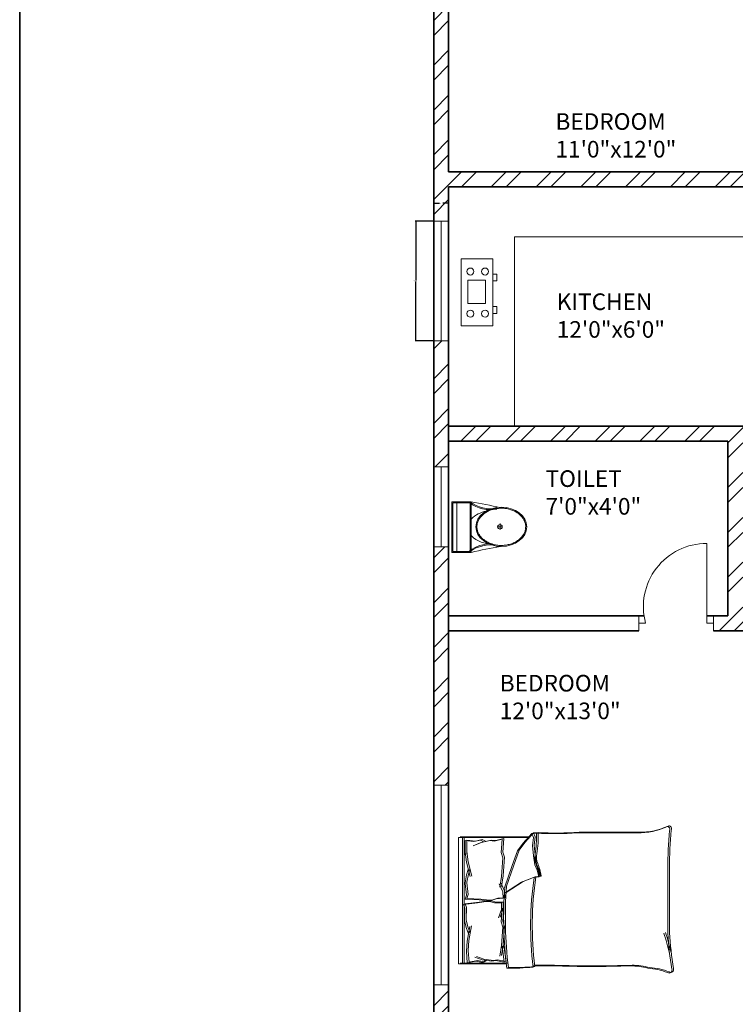
# Model space of a CAD drawing. Units: inches. Extents: x 1962 to 2771, y 1245 to 2660.
# Tile 2 of 114: x 1962 to 2177, y 1534 to 1831. Entities that reach past the tile are written whole.
import ezdxf

# ---------------------------------------------------------------- set-up
doc = ezdxf.new("R2010")
doc.units = ezdxf.units.IN
for name, color, linetype, lineweight in [('A-ANNO-DIMS', 2, 'Continuous', 18), ('A-ANNO-TTLB', 7, 'Continuous', 35), ('A-AREA-IDEN', 7, 'Continuous', 18), ('A-DOOR', 3, 'Continuous', 18), ('A-EQPM', 8, 'Continuous', 18), ('A-FLOR-CASE', 8, 'Continuous', 18), ('A-FLOR-FIXT', 8, 'Continuous', 18), ('A-FURN', 8, 'Continuous', 13), ('A-GLAZ', 4, 'Continuous', 18), ('A-WALL', 7, 'Continuous', 35), ('A-WALL-PATT', 252, 'Continuous', 13)]:
    doc.layers.add(name, color=color, linetype=linetype, lineweight=lineweight)
doc.styles.get("Standard").update_dxf_attribs({"font": 'arial.ttf'})
doc.dimstyles.get("Standard").update_dxf_attribs({"dimtxt": 0.18, "dimasz": 0.18, "dimexe": 0.18, "dimexo": 0.0625, "dimgap": 0.09, "dimtad": 0, "dimtih": 1, "dimtoh": 1, "dimdec": 4, "dimzin": 0, "dimdsep": 46, "dimtxsty": 'Standard', "dimcen": 0.09, "dimadec": 0, "dimazin": 0, "dimtfac": 1, "dimtdec": 4, "dimtofl": 0, "dimtmove": 0, "dimatfit": 3, "dimfxl": 1, "dimtolj": 1, "dimtzin": 0, "dimarcsym": 0})

# ---------------------------------------------------------------- blocks, each defined once
blk = doc.blocks.new('A$C31115884')
for p, q in [((258, 466), (258, 523)), ((283, 498), (223, 498)), ((0, 200), (0, 0)), ((520, 200), (0, 200)), ((10, 190), (10, 10)), ((510, 190), (10, 190)), ((510, 10), (510, 190)), ((520, 0), (520, 200)), ((510, 54), (0, 54)), ((10, 10), (510, 10)), ((0, 0), (520, 0))]:
    blk.add_line(p, q)
blk.add_circle((256, 496), 23.6)
for centre, radius, start, end in [((2778, -205), 2807, 165.4549, 171.7133), ((-295, 403), 365, 324.2091, 9.3499), ((-295, 403), 375, 324.2091, 9.3499), ((139, 406), 293, 315.8436, 2.6563), ((806, 403), 375, 179.2036, 215.7909), ((806, 403), 365, 170.6501, 215.7909), ((3237, 905), 2807, 188.2867, 194.5451), ((384, 406), 293, 190.2774, 224.1564)]:
    blk.add_arc(centre, radius, start, end)
blk.add_ellipse((256, 510), major_axis=(0, -261), ratio=0.772727)
blk.add_open_spline([(256, 259), (263, 259), (270, 260), (288, 262), (299, 265), (320, 273), (330, 278), (350, 291), (360, 299), (378, 316), (386, 326), (402, 347), (409, 358), (421, 383), (427, 395), (436, 422), (440, 436), (445, 465), (447, 480), (448, 509), (448, 524), (445, 553), (443, 568), (436, 596), (432, 610), (422, 636), (416, 649), (402, 672), (395, 683), (379, 703), (370, 712), (351, 728), (341, 735), (321, 746), (310, 751), (289, 757), (278, 759), (256, 761), (245, 761), (223, 757), (212, 754), (191, 746), (181, 741), (161, 728), (151, 720), (133, 703), (125, 693), (110, 672), (103, 660), (90, 636), (85, 623), (76, 596), (72, 582), (67, 553), (66, 538), (64, 509), (65, 494), (68, 465), (70, 450), (77, 422), (81, 408), (91, 382), (97, 370), (111, 346), (118, 335), (135, 316), (144, 307), (162, 291), (172, 284), (193, 273), (203, 269), (225, 262), (236, 260), (250, 259), (253, 259), (256, 259)], degree=3, knots=[0, 0, 0, 0, 0.110105, 0.110105, 0.285049, 0.285049, 0.459994, 0.459994, 0.634938, 0.634938, 0.809882, 0.809882, 0.984827, 0.984827, 1.159771, 1.159771, 1.334715, 1.334715, 1.50966, 1.50966, 1.684604, 1.684604, 1.859549, 1.859549, 2.034493, 2.034493, 2.209437, 2.209437, 2.384382, 2.384382, 2.559326, 2.559326, 2.73427, 2.73427, 2.909215, 2.909215, 3.084159, 3.084159, 3.259103, 3.259103, 3.434048, 3.434048, 3.608992, 3.608992, 3.783936, 3.783936, 3.958881, 3.958881, 4.133825, 4.133825, 4.30877, 4.30877, 4.483714, 4.483714, 4.658658, 4.658658, 4.833603, 4.833603, 5.008547, 5.008547, 5.183491, 5.183491, 5.358436, 5.358436, 5.53338, 5.53338, 5.708324, 5.708324, 5.883269, 5.883269, 6.058213, 6.058213, 6.233158, 6.233158, 6.283185, 6.283185, 6.283185, 6.283185])
blk = doc.blocks.new('BED-PLAN')
for p, q in [((22.05, 42.03), (19.47, 39.08)), ((22.05, 42.02), (19.47, 39.08)), ((22.56, 42.21), (19.98, 39.26)), ((22.56, 42.21), (19.98, 39.26)), ((23.44, 42.09), (22.05, 42.03, 3.08)), ((23.44, 42.09), (22.05, 42.02, 3.08)), ((22.55, 40.8), (22.05, 42.03)), ((22.55, 40.8), (22.05, 42.02)), ((23.95, 42.27), (22.56, 42.21, 3.08)), ((23.95, 42.27), (22.56, 42.21, 3.08)), ((23.06, 40.98), (22.56, 42.21)), ((23.06, 40.98), (22.56, 42.21)), ((0, 40.75), (21.15, 40.75)), ((0, 40.75), (21.15, 40.75)), ((0, 2.76), (0, 40.75)), ((0.51, 40.93), (21.66, 40.93)), ((0.51, 40.93), (21.66, 40.93)), ((1.22, 2.76), (1.22, 40.75)), ((1.22, 2.76), (1.22, 40.75)), ((1.73, 2.95), (1.73, 40.93)), ((1.73, 2.95), (1.73, 40.93)), ((2.03, 39.83), (1.96, 35.54)), ((2.03, 39.83), (1.96, 35.54)), ((2.03, 39.83), (4.58, 39.53)), ((2.03, 39.83), (4.58, 39.53)), ((2.54, 40.02), (2.46, 35.72)), ((2.54, 40.02), (2.46, 35.72)), ((2.54, 40.02), (5.09, 39.72)), ((2.54, 40.02), (5.09, 39.72)), ((6.56, 39.2), (4.43, 38.26)), ((6.56, 39.2), (4.43, 38.26)), ((4.58, 39.53), (6.63, 40.01)), ((4.58, 39.53), (6.63, 40.01)), ((7.07, 39.38), (4.94, 38.44)), ((7.07, 39.38), (4.94, 38.44)), ((5.09, 39.72), (7.14, 40.19)), ((5.09, 39.72), (7.14, 40.19)), ((9.4, 39.83), (6.56, 39.2)), ((9.4, 39.83), (6.56, 39.2)), ((6.63, 40.01), (7.46, 39.6)), ((6.63, 40.01), (7.46, 39.6)), ((9.91, 40.02), (7.07, 39.38)), ((9.91, 40.02), (7.07, 39.38)), ((7.14, 40.19), (7.97, 39.78)), ((7.14, 40.19), (7.97, 39.78)), ((10.68, 39.68), (9.4, 39.83)), ((10.68, 39.68), (9.4, 39.83)), ((11.19, 39.87), (9.91, 40.02)), ((11.19, 39.87), (9.91, 40.02)), ((13.17, 40.3), (10.68, 39.68)), ((13.17, 40.3), (10.68, 39.68)), ((13.68, 40.48), (11.19, 39.87)), ((13.68, 40.48), (11.19, 39.87)), ((12.85, 36.22), (13.17, 40.3)), ((12.85, 36.22), (13.17, 40.3)), ((13.36, 36.4), (13.68, 40.48)), ((13.36, 36.4), (13.68, 40.48)), ((19.47, 39.08), (17.75, 36.74)), ((19.47, 39.08), (17.75, 36.74)), ((19.98, 39.26), (18.26, 36.92)), ((19.98, 39.26), (18.26, 36.92)), ((22.3, 38.34), (22.55, 40.8)), ((22.3, 38.34), (22.55, 40.8)), ((22.81, 38.52), (23.06, 40.98)), ((22.81, 38.52), (23.06, 40.98)), ((23.06, 35.45), (22.81, 38.52)), ((23.06, 35.44), (22.81, 38.52)), ((1.96, 35.54), (2.02, 36.34)), ((1.96, 35.54), (2.02, 36.34)), ((2.02, 36.34), (2.44, 33.32)), ((2.02, 36.34), (2.44, 33.32)), ((2.46, 35.72), (2.53, 36.52)), ((2.46, 35.72), (2.53, 36.52)), ((2.53, 36.52), (2.95, 33.5)), ((2.53, 36.52), (2.95, 33.5)), ((13.3, 34.66), (12.85, 36.22)), ((13.3, 34.66), (12.85, 36.22)), ((13.8, 34.84), (13.36, 36.4)), ((13.8, 34.84), (13.36, 36.4)), ((17.75, 36.74), (16.15, 32.31)), ((17.75, 36.74), (16.15, 32.31)), ((18.26, 36.92), (16.66, 32.49)), ((18.26, 36.92), (16.66, 32.49)), ((22.55, 35.26), (22.3, 38.34)), ((22.55, 35.26), (22.3, 38.34)), ((2.44, 33.32), (3.52, 29.01)), ((2.44, 33.32), (3.52, 29.01)), ((2.95, 33.5), (4.02, 29.19)), ((2.95, 33.5), (4.02, 29.19)), ((12.95, 29.09), (13.3, 34.66)), ((12.95, 29.09), (13.3, 34.66)), ((13.46, 29.27), (13.8, 34.84)), ((13.46, 29.27), (13.8, 34.84)), ((22.92, 32.56), (22.55, 35.26)), ((22.92, 32.55), (22.55, 35.26)), ((23.42, 32.74), (23.06, 35.45)), ((23.42, 32.74), (23.06, 35.44)), ((24.16, 31.14), (23.42, 32.74)), ((24.16, 31.14), (23.42, 32.74)), ((2.92, 31.16), (2.45, 29.52)), ((2.92, 31.16), (2.45, 29.52)), ((2.96, 29.7), (2.52, 27.37)), ((2.96, 29.7), (2.52, 27.37)), ((3.43, 31.34), (2.96, 29.7)), ((3.43, 31.34), (2.96, 29.7)), ((16.15, 32.31), (13.82, 25.68)), ((16.15, 32.31), (13.82, 25.68)), ((16.66, 32.49), (14.33, 25.86)), ((16.66, 32.49), (14.33, 25.86)), ((23.65, 30.95), (22.92, 32.56)), ((23.65, 30.95), (22.92, 32.55)), ((24.15, 28.99), (23.65, 30.95)), ((24.15, 28.98), (23.65, 30.95)), ((24.65, 29.17), (24.16, 31.14)), ((24.65, 29.17), (24.16, 31.14)), ((62.99, 11.98), (62.99, 31.54)), ((62.99, 11.97), (62.99, 31.54)), ((63.5, 12.16), (63.5, 31.72)), ((63.5, 12.16), (63.5, 31.72)), ((2.45, 29.52), (2.02, 27.19)), ((2.45, 29.52), (2.02, 27.19)), ((2.02, 27.19), (2.03, 26.94)), ((2.02, 27.19), (2.03, 26.93)), ((2.03, 26.94), (2.37, 23.42)), ((2.03, 26.93), (2.37, 23.42)), ((2.52, 27.37), (2.54, 27.12)), ((2.52, 27.37), (2.54, 27.12)), ((2.54, 27.12), (2.88, 23.6)), ((2.54, 27.12), (2.88, 23.6)), ((13.31, 24.44), (12.28, 26.89)), ((13.31, 24.44), (12.28, 26.88)), ((12.42, 25.89), (12.95, 29.09)), ((12.42, 25.89), (12.95, 29.09)), ((13.81, 24.63), (12.79, 27.07)), ((13.81, 24.63), (12.79, 27.07)), ((12.93, 26.07), (13.46, 29.27)), ((12.93, 26.07), (13.46, 29.27)), ((13.82, 24.05), (18.98, 27.38)), ((13.82, 24.05), (18.98, 27.38)), ((14.33, 24.24), (19.49, 27.57)), ((14.33, 24.24), (19.49, 27.57)), ((18.98, 27.38), (22.55, 28.74)), ((18.98, 27.38), (22.55, 28.74)), ((19.49, 27.57), (23.06, 28.92)), ((19.49, 27.57), (23.06, 28.92)), ((22.55, 28.74), (24.15, 28.99)), ((22.55, 28.74), (24.15, 28.98)), ((23.06, 28.92), (24.65, 29.17)), ((23.06, 28.92), (24.65, 29.17)), ((13.43, 22.49), (13.31, 24.44)), ((13.43, 22.49), (13.31, 24.44)), ((13.94, 22.68), (13.81, 24.63)), ((13.94, 22.68), (13.81, 24.63)), ((1.49, 20.65), (5.74, 21.11)), ((1.49, 20.65), (5.74, 21.11)), ((2.37, 23.42), (1.98, 22.24)), ((2.37, 23.42), (1.98, 22.24)), ((1.98, 22.24), (6.25, 22.05)), ((1.98, 22.24), (6.25, 22.05)), ((1.99, 20.84), (6.25, 21.3)), ((1.99, 20.84), (6.25, 21.3)), ((2.45, 19.69), (1.99, 20.84)), ((2.45, 19.69), (1.99, 20.84)), ((2.88, 23.6), (2.49, 22.42)), ((2.88, 23.6), (2.49, 22.42)), ((2.49, 22.42), (6.76, 22.23)), ((2.49, 22.42), (6.76, 22.23)), ((5.74, 21.11), (8.27, 21.57)), ((5.74, 21.11), (8.27, 21.57)), ((6.25, 22.05), (8.81, 21.75)), ((6.25, 22.05), (8.81, 21.75)), ((6.25, 21.3), (8.78, 21.76)), ((6.25, 21.3), (8.78, 21.76)), ((6.76, 22.23), (9.31, 21.93)), ((6.76, 22.23), (9.31, 21.93)), ((8.27, 21.57), (9.3, 21.57)), ((8.27, 21.57), (9.3, 21.57)), ((8.78, 21.76), (9.81, 21.76)), ((8.78, 21.76), (9.81, 21.76)), ((8.81, 21.75), (9.84, 21.81)), ((8.81, 21.75), (9.84, 21.81)), ((9.3, 21.57), (10.8, 21.11)), ((9.3, 21.57), (10.8, 21.11)), ((9.31, 21.93), (10.35, 21.99)), ((9.31, 21.93), (10.35, 21.99)), ((9.81, 21.76), (11.3, 21.3)), ((9.81, 21.76), (11.3, 21.3)), ((9.84, 21.81), (11.3, 22.36)), ((9.84, 21.81), (11.3, 22.36)), ((10.35, 21.99), (11.81, 22.54)), ((10.35, 21.99), (11.81, 22.54)), ((10.8, 21.11), (12.93, 21.11)), ((10.8, 21.11), (12.93, 21.11)), ((11.3, 22.36), (13.43, 22.49)), ((11.3, 22.36), (13.43, 22.49)), ((11.3, 21.3), (13.44, 21.3)), ((11.3, 21.3), (13.44, 21.3)), ((11.81, 22.54), (13.94, 22.68)), ((11.81, 22.54), (13.94, 22.68)), ((12.93, 21.11), (12.93, 19.16)), ((12.93, 21.11), (12.93, 19.16)), ((13.44, 21.3), (13.44, 19.34)), ((13.44, 21.3), (13.44, 19.34)), ((1.95, 19.51), (1.49, 20.65)), ((1.95, 19.51), (1.49, 20.65)), ((1.83, 15.97), (1.95, 19.51)), ((1.83, 15.97), (1.95, 19.51)), ((2.34, 16.15), (2.45, 19.69)), ((2.34, 16.15), (2.45, 19.69)), ((12.93, 19.16), (12.06, 16.66)), ((12.93, 19.16), (12.06, 16.66)), ((13.44, 19.34), (12.57, 16.84)), ((13.44, 19.34), (12.57, 16.84)), ((12.85, 15.41), (13.17, 19.49)), ((12.85, 15.41), (13.17, 19.49)), ((13.36, 15.59), (13.68, 19.67)), ((13.36, 15.59), (13.68, 19.67)), ((1.83, 15.72), (1.83, 15.97)), ((1.83, 15.72), (1.83, 15.97)), ((2.41, 13.42), (1.83, 15.72)), ((2.41, 13.42), (1.83, 15.72)), ((2.34, 15.9), (2.34, 16.15)), ((2.34, 15.9), (2.34, 16.15)), ((2.91, 13.6), (2.34, 15.9)), ((2.91, 13.6), (2.34, 15.9)), ((13.3, 13.85), (12.85, 15.41)), ((13.3, 13.85), (12.85, 15.41)), ((13.8, 14.03), (13.36, 15.59)), ((13.8, 14.03), (13.36, 15.59)), ((2.98, 11.81), (2.41, 13.42)), ((2.98, 11.81), (2.41, 13.42)), ((2.64, 9.63), (3.44, 13.99)), ((2.64, 9.63), (3.44, 13.99)), ((3.49, 11.99), (2.91, 13.6)), ((3.49, 11.99), (2.91, 13.6)), ((3.14, 9.81), (3.95, 14.17)), ((3.14, 9.81), (3.95, 14.17)), ((12.95, 8.28), (13.3, 13.85)), ((12.95, 8.28), (13.3, 13.85)), ((13.46, 8.46), (13.8, 14.03)), ((13.46, 8.46), (13.8, 14.03)), ((2.41, 6.59), (2.64, 9.63)), ((2.41, 6.59), (2.64, 9.63)), ((2.91, 6.77), (3.14, 9.81)), ((2.91, 6.77), (3.14, 9.81)), ((2.39, 6.5), (2.41, 6.59)), ((2.39, 6.5), (2.41, 6.59)), ((2.65, 3.1), (2.39, 6.5)), ((2.65, 3.1), (2.39, 6.5)), ((2.9, 6.68), (2.91, 6.77)), ((2.9, 6.68), (2.91, 6.77)), ((3.16, 3.28), (2.9, 6.68)), ((3.16, 3.28), (2.9, 6.68)), ((12.42, 5.07), (12.95, 8.28)), ((12.42, 5.07), (12.95, 8.28)), ((12.93, 5.26), (13.46, 8.46)), ((12.93, 5.26), (13.46, 8.46)), ((12.95, 8.28), (13.21, 7.38)), ((12.95, 8.28), (13.21, 7.38)), ((13.21, 7.38), (13.78, 3.33)), ((13.21, 7.38), (13.78, 3.33)), ((13.46, 8.46), (13.72, 7.56)), ((13.46, 8.46), (13.72, 7.56)), ((13.72, 7.56), (14.29, 3.51)), ((13.72, 7.56), (14.29, 3.51)), ((2.64, 3.1), (5.16, 3.56)), ((2.64, 3.1), (5.16, 3.56)), ((3.14, 3.28), (5.67, 3.74)), ((3.14, 3.28), (5.67, 3.74)), ((7.12, 4.02), (4.93, 4.82)), ((7.12, 4.02), (4.93, 4.82)), ((5.16, 3.56), (7.23, 3.21)), ((5.16, 3.56), (7.23, 3.21)), ((7.63, 4.2), (5.44, 5)), ((7.63, 4.2), (5.44, 5)), ((5.67, 3.74), (7.74, 3.39)), ((5.67, 3.74), (7.74, 3.39)), ((9.99, 3.56), (7.12, 4.02)), ((9.99, 3.56), (7.12, 4.02)), ((7.23, 3.21), (8.04, 3.67)), ((7.23, 3.21), (8.04, 3.67)), ((10.5, 3.74), (7.63, 4.2)), ((10.5, 3.74), (7.63, 4.2)), ((7.74, 3.39), (8.55, 3.85)), ((7.74, 3.39), (8.55, 3.85)), ((11.26, 3.79), (9.99, 3.56)), ((11.26, 3.79), (9.99, 3.56)), ((11.76, 3.97), (10.5, 3.74)), ((11.76, 3.97), (10.5, 3.74)), ((13.78, 3.33), (11.26, 3.79)), ((13.78, 3.33), (11.26, 3.79)), ((14.29, 3.51), (11.76, 3.97)), ((14.29, 3.51), (11.76, 3.97)), ((14.4, 2.76), (0, 2.76)), ((14.4, 2.76), (0, 2.76)), ((14.9, 2.95), (0.51, 2.95)), ((14.9, 2.95), (0.51, 2.95))]:
    blk.add_line(p, q)
for centre, radius, start, end in [((-5.29, 40.8), 28.76, 349.8763, 2.5657), ((-5.29, 40.8), 28.76, 349.8763, 2.5657), ((28.87, 144.88), 102.94, 266.9791, 273.8365), ((28.87, 144.88), 102.94, 266.9791, 273.8365), ((-4.78, 40.98), 28.76, 349.8763, 2.5657), ((-4.78, 40.98), 28.76, 349.8763, 2.5657), ((29.37, 145.06), 102.94, 266.9791, 273.8365), ((29.37, 145.06), 102.94, 266.9791, 273.8365), ((53.91, -3583.94), 3626.16, 90.00217, 90.28689), ((53.91, -3583.94), 3626.16, 90.00217, 90.28689), ((54.42, -3583.75), 3626.16, 90.00217, 90.28689), ((54.42, -3583.75), 3626.16, 90.00217, 90.28689), ((54.58, 60.54), 18.33, 267.4714, 296.4681), ((54.58, 60.54), 18.33, 267.4714, 296.4681), ((55.09, 60.72), 18.33, 267.4714, 296.4681), ((55.09, 60.72), 18.33, 267.4714, 296.4681), ((62.69, 43.25), 0.876, 332.6588, 86.02), ((62.69, 43.25), 0.876, 332.6588, 86.02), ((168.74, 32.71), 105.75, 174.4998, 180.6351), ((168.74, 32.71), 105.75, 174.4998, 180.6351), ((63.2, 43.43), 0.876, 332.6588, 86.02), ((63.2, 43.43), 0.876, 332.6588, 86.02), ((169.24, 32.89), 105.75, 174.4998, 180.6351), ((169.24, 32.89), 105.75, 174.4998, 180.6351), ((27.87, 34.77), 4.95, 168.6608, 203.7384), ((27.87, 34.77), 4.95, 168.6608, 203.7384), ((28.38, 34.95), 4.95, 168.6608, 203.7384), ((28.38, 34.95), 4.95, 168.6608, 203.7384), ((1.18, 24.77), 23.57, 10.6617, 19.8806), ((1.18, 24.76), 23.57, 10.6617, 19.8806), ((1.69, 24.95), 23.57, 10.6617, 19.8806), ((1.69, 24.95), 23.57, 10.6617, 19.8806), ((124.25, 14.12), 102.56, 171.7845, 186.9006), ((124.25, 14.11), 102.56, 171.7845, 186.9006), ((124.76, 14.3), 102.56, 171.7845, 186.9006), ((124.76, 14.3), 102.56, 171.7845, 186.9006), ((24.2, 29.12), 0.147, 250.2464, 1.1377), ((24.2, 29.12), 0.147, 250.2464, 1.1377), ((24.7, 29.3), 0.147, 250.2464, 1.1377), ((24.7, 29.3), 0.147, 250.2464, 1.1377), ((144.71, 16.98), 131.13, 176.0865, 186.7821), ((144.71, 16.98), 131.13, 176.0865, 186.7821), ((145.22, 17.16), 131.13, 176.0865, 186.7821), ((145.22, 17.16), 131.13, 176.0865, 186.7821), ((-18.85, -13.69), 84.62, 13.3832, 17.7053), ((-18.85, -13.69), 84.62, 13.3832, 17.7053), ((-18.34, -13.51), 84.62, 13.3832, 17.7053), ((-18.34, -13.51), 84.62, 13.3832, 17.7053), ((159.64, 17.03), 96.78, 182.9958, 189.4091), ((159.64, 17.03), 96.78, 182.9958, 189.4091), ((160.15, 17.21), 96.78, 182.9958, 189.4091), ((160.15, 17.21), 96.78, 182.9958, 189.4091), ((15.97, 67.7), 66.22, 268.7218, 275.604), ((15.97, 67.7), 66.22, 268.7218, 275.604), ((16.48, 67.88), 66.22, 268.7218, 275.604), ((16.48, 67.88), 66.22, 268.7218, 275.604), ((24.78, -132.99), 135.22, 88.4762, 91.0082), ((24.78, -132.99), 135.22, 88.4762, 91.0082), ((25.29, -132.81), 135.22, 88.4762, 91.0082), ((25.29, -132.81), 135.22, 88.4762, 91.0082), ((40.23, 385.38), 383.38, 268.2277, 271.7185), ((40.23, 385.38), 383.38, 268.2277, 271.7185), ((40.74, 385.56), 383.38, 268.2277, 271.7185), ((40.74, 385.56), 383.38, 268.2277, 271.7185), ((51.28, -21.38), 23.56, 76.0648, 88.9113), ((51.28, -21.38), 23.56, 76.0648, 88.9113), ((51.79, -21.2), 23.56, 76.0648, 88.9113), ((51.79, -21.2), 23.56, 76.0648, 88.9113), ((55.86, -17.22), 18.73, 67.9751, 86.652), ((55.86, -17.22), 18.73, 67.9751, 86.652), ((56.37, -17.03), 18.73, 67.9751, 86.652), ((56.37, -17.03), 18.73, 67.9751, 86.652), ((63.37, 0.87), 0.866, 236.1736, 23.4781), ((63.37, 0.87), 0.866, 236.1736, 23.4781), ((63.87, 1.05), 0.866, 236.1736, 23.4781), ((63.87, 1.05), 0.866, 236.1736, 23.4781)]:
    blk.add_arc(centre, radius, start, end)
blk = doc.blocks.new('COOKTOP-4-BURNER')
for points in [[(0, 20.18), (9.48, 20.18), (9.48, 0), (0, 0)], [(9.48, 15.59), (10.71, 15.59), (10.71, 13.59), (9.48, 13.59)], [(2, 13.79), (7.26, 13.79), (7.26, 6.73), (2, 6.73)], [(9.48, 5.81), (10.71, 5.81), (10.71, 3.8), (9.48, 3.8)]]:
    blk.add_lwpolyline(points, close=True)
for centre in [(2.74, 16.38), (7.14, 16.38), (2.74, 3.71), (7.14, 3.71)]:
    blk.add_circle(centre, 1.05)
blk = doc.blocks.new('WIN-24IN-B')
for p, q in [((0, 24), (4.5, 24)), ((4.5, 24), (2.25, 24)), ((2.25, 24), (2.25, 0)), ((4.5, 0), (0, 0)), ((2.25, 0), (4.5, 0))]:
    blk.add_line(p, q)
blk = doc.blocks.new('WIN-60IN-B')
for p, q in [((0, 60), (4.5, 60)), ((4.5, 60), (2.25, 60)), ((2.25, 60), (2.25, 0)), ((4.5, 0), (0, 0)), ((2.25, 0), (4.5, 0))]:
    blk.add_line(p, q)
blk = doc.blocks.new('WIN-36IN-A')
for p, q in [((4.5, 36), (0, 36)), ((0, 36), (2.25, 36)), ((2.25, 36), (2.25, 0)), ((2.25, 0), (0, 0)), ((0, 0), (4.5, 0))]:
    blk.add_line(p, q)
blk = doc.blocks.new('*D26')
at = {"layer": 'A-ANNO-DIMS', "color": 0, "lineweight": -2, "transparency": 16777216}
for p, q in [((2086.24, 1769.99), (2080.73, 1769.99)), ((2080.91, 1769.81), (2080.91, 1752.17)), ((2080.91, 1734.17), (2080.91, 1751.81)), ((2086.24, 1733.99), (2080.73, 1733.99))]:
    blk.add_line(p, q, dxfattribs=at)
at = {"layer": 'A-ANNO-DIMS', "color": 0, "transparency": 16777216}
for points in [[(2080.88, 1769.81), (2080.94, 1769.81), (2080.91, 1769.99)], [(2080.88, 1734.17), (2080.94, 1734.17), (2080.91, 1733.99)]]:
    blk.add_solid(points, dxfattribs=at)
at = {"layer": 'Defpoints', "color": 0, "transparency": 16777216}
for p in [(2080.91, 1769.99), (2086.31, 1769.99), (2086.31, 1733.99)]:
    blk.add_point(p, dxfattribs=at)
at = {"layer": 'A-ANNO-DIMS', "color": 0, "transparency": 16777216, "insert": (2080.91, 1751.99), "char_height": 0.18, "attachment_point": 5}
blk.add_mtext('\\A1;W2A 36 TYP.', dxfattribs=at)
blk = doc.blocks.new('*D27')
at = {"layer": 'A-ANNO-DIMS', "color": 0, "lineweight": -2, "transparency": 16777216}
for p, q in [((2086.31, 1770.05), (2086.31, 1775.57)), ((2086.49, 1775.39), (2088.1, 1775.39)), ((2090.63, 1775.39), (2089.02, 1775.39)), ((2090.81, 1770.05), (2090.81, 1775.57))]:
    blk.add_line(p, q, dxfattribs=at)
at = {"layer": 'A-ANNO-DIMS', "color": 0, "transparency": 16777216}
for points in [[(2086.49, 1775.42), (2086.49, 1775.36), (2086.31, 1775.39)], [(2090.63, 1775.42), (2090.63, 1775.36), (2090.81, 1775.39)]]:
    blk.add_solid(points, dxfattribs=at)
at = {"layer": 'Defpoints', "color": 0, "transparency": 16777216}
for p in [(2090.81, 1775.39), (2086.31, 1769.99), (2090.81, 1769.99)]:
    blk.add_point(p, dxfattribs=at)
at = {"layer": 'A-ANNO-DIMS', "color": 0, "transparency": 16777216, "insert": (2088.56, 1775.39), "char_height": 0.18, "attachment_point": 5}
blk.add_mtext('\\A1;5 TYP.', dxfattribs=at)

msp = doc.modelspace()

# ---------------------------------------------------------------- hatches: boundary and pattern name
at = {"layer": 'A-WALL-PATT'}
h = msp.add_hatch(dxfattribs=at)
h.set_pattern_fill('ANSI32', color=256)
h.paths.add_polyline_path([(2090.8074, 2467.3437), (2141.6481, 2467.3437), (2141.6481, 2469.5937), (2141.6481, 2471.8437), (2086.3074, 2471.8437), (2086.3074, 2422.5333), (2090.8074, 2422.5333)])
h.paths.add_polyline_path([(2282.7664, 2471.8437), (2204.8982, 2471.8437), (2204.8982, 2467.3437), (2234.8074, 2467.3437), (2234.8074, 2311.3437), (2228.7492, 2311.3437), (2228.7492, 2306.8437), (2234.8074, 2306.8437), (2331.9227, 2306.8437), (2331.9227, 2309.0937), (2331.9227, 2311.3437), (2239.3074, 2311.3437), (2239.3074, 2467.3437), (2282.7664, 2467.3437), (2282.7664, 2469.5937)])
h.paths.add_polyline_path([(2471.4531, 2519.8437), (2552.011, 2519.8437), (2564.3996, 2519.8437), (2564.3996, 2511.1389), (2568.8996, 2511.1389), (2568.8996, 2524.3437), (2466.9531, 2524.3437), (2466.9531, 2471.8437), (2450.0749, 2471.8437), (2446.4672, 2471.8437), (2446.4672, 2467.3437), (2450.0749, 2467.3437), (2475.9988, 2467.3437), (2475.9988, 2469.5937), (2475.9988, 2471.8437), (2471.4531, 2471.8437)])
h.paths.add_polyline_path([(2575.2231, 2469.5937), (2575.2231, 2471.8437), (2568.8996, 2471.8437), (2568.8996, 2487.1389), (2564.3996, 2487.1389), (2564.3996, 2471.8437), (2556.511, 2471.8437), (2499.2904, 2471.8437), (2499.2904, 2467.3437), (2507.8074, 2467.3437), (2507.8074, 2311.3437), (2414.863, 2311.3437), (2414.863, 2306.8437), (2512.3074, 2306.8437), (2517.0114, 2306.8437), (2517.0114, 2309.0937), (2517.0114, 2311.3437), (2512.3074, 2311.3437), (2512.3074, 2467.3437), (2575.2231, 2467.3437)])
h.paths.add_polyline_path([(2660.8074, 2471.8437), (2600.9602, 2471.8437), (2600.9602, 2467.3437), (2656.3074, 2467.3437), (2656.3074, 2432.5704), (2660.8074, 2432.5704)])
h.paths.add_polyline_path([(2660.8074, 2372.5704), (2656.3074, 2372.5704), (2656.3074, 2311.3437), (2600.276, 2311.3437), (2600.276, 2309.0937), (2600.276, 2306.8437), (2656.3074, 2306.8437), (2656.3074, 2296.2593), (2660.8074, 2296.2593)])
h.paths.add_polyline_path([(2572.3074, 2306.8437), (2577.1385, 2306.8437), (2577.1385, 2311.3437), (2551.082, 2311.3437), (2551.082, 2306.8437), (2567.8074, 2306.8437), (2567.8074, 2258.8437), (2540.0574, 2258.8437), (2540.0574, 2256.5937), (2540.0574, 2254.3437), (2567.8074, 2254.3437), (2656.3074, 2254.3437), (2656.3074, 2236.9085), (2660.8074, 2236.9085), (2660.8074, 2272.2593), (2656.3074, 2272.2593), (2656.3074, 2258.8437), (2572.3074, 2258.8437)])
h.paths.add_polyline_path([(2512.3074, 2254.3437), (2518.8716, 2254.3437), (2518.8716, 2256.5937), (2518.8716, 2258.8437), (2507.8074, 2258.8437), (2507.8074, 2177.8437), (2567.8074, 2177.8437), (2567.8074, 2172.9628), (2572.3074, 2172.9628), (2572.3074, 2177.8437), (2656.3074, 2177.8437), (2656.3074, 2166.4846), (2660.8074, 2166.4846), (2660.8074, 2200.9085), (2656.3074, 2200.9085), (2656.3074, 2182.3437), (2512.3074, 2182.3437)])
h.paths.add_polyline_path([(2656.3074, 2129.8437), (2572.3074, 2129.8437), (2572.3074, 2150.3044), (2570.0574, 2150.3044), (2567.8074, 2150.3044), (2567.8074, 2129.8437), (2507.8074, 2129.8437), (2507.8074, 2116.3027), (2510.0574, 2116.3027), (2512.3074, 2116.3027), (2512.3074, 2125.3437), (2567.8074, 2125.3437), (2572.3074, 2125.3437), (2656.3074, 2125.3437)])
h.paths.add_polyline_path([(2090.8074, 2362.5333), (2086.3074, 2362.5333), (2086.3074, 2298.6242), (2090.8074, 2298.6242), (2090.8074, 2306.8437), (2174.8074, 2306.8437), (2174.8074, 2286.4178), (2179.3074, 2286.4178), (2179.3074, 2306.8437), (2192.8641, 2306.8437), (2192.8641, 2309.0937), (2192.8641, 2311.3437), (2090.8074, 2311.3437)])
h.paths.add_polyline_path([(2209.156, 2258.8437), (2179.3074, 2258.8437), (2179.3074, 2263.2236), (2177.0574, 2263.2236), (2174.8074, 2263.2236), (2174.8074, 2258.8437), (2090.8074, 2258.8437), (2090.8074, 2274.6242), (2086.3074, 2274.6242), (2086.3074, 2238.2967), (2088.5574, 2238.2967), (2090.8074, 2238.2967), (2090.8074, 2254.3437), (2209.156, 2254.3437)])
h.paths.add_polyline_path([(2090.8074, 2177.8437), (2234.8074, 2177.8437), (2234.8074, 2173.1428), (2239.3074, 2173.1428), (2239.3074, 2258.8437), (2230.8442, 2258.8437), (2230.8442, 2256.5937), (2230.8442, 2254.3437), (2234.8074, 2254.3437), (2234.8074, 2182.3437), (2090.8074, 2182.3437), (2090.8074, 2202.2967), (2086.3074, 2202.2967), (2086.3074, 2140.0389), (2090.8074, 2140.0389)])
h.paths.add_polyline_path([(2090.8074, 2080.0389), (2086.3074, 2080.0389), (2086.3074, 2033.8437), (2090.8074, 2033.8437)], flags=17)
h.paths.add_polyline_path([(2244.9405, 2033.8437), (2239.3074, 2033.8437), (2239.3074, 2142.0665), (2237.2592, 2142.0665), (2234.8074, 2142.0665), (2234.8074, 2033.8437), (2090.8074, 2033.8437), (2076.5204, 2033.8437), (2072.0204, 2033.8437), (2072.0204, 2000.4493), (2076.5204, 2000.4493), (2076.5204, 2029.3437), (2090.8074, 2029.3437), (2244.9405, 2029.3437), (2244.9405, 2031.5937)])
h.paths.add_polyline_path([(2234.8074, 1933.3437), (2076.5204, 1933.3437), (2076.5204, 1952.4493), (2074.2704, 1952.4493), (2072.0204, 1952.4493), (2072.0204, 1933.3437), (2072.0204, 1928.8437), (2234.8074, 1928.8437)])
h.paths.add_polyline_path([(2090.8074, 1928.8437), (2086.3074, 1928.8437), (2086.3074, 1906.5013), (2090.8074, 1906.5013)])
h.paths.add_polyline_path([(2090.8074, 1846.5013), (2086.3074, 1846.5013), (2086.3074, 1769.9917), (2088.5574, 1769.9917), (2090.8074, 1769.9917), (2090.8074, 1780.3437), (2234.8074, 1780.3437), (2234.8074, 1708.3437), (2230.3764, 1708.3437), (2230.3764, 1703.8437), (2239.3074, 1703.8437), (2239.3074, 1792.6669), (2237.0574, 1792.6669), (2234.8074, 1792.6669), (2234.8074, 1784.8437), (2090.8074, 1784.8437)])
h.paths.add_polyline_path([(2239.3074, 1928.8437), (2244.9405, 1928.8437), (2244.9405, 1931.0937), (2244.9405, 1933.3437), (2234.8074, 1933.3437), (2234.8074, 1928.8437), (2234.8074, 1825.5949), (2239.3074, 1825.5949)])
h.paths.add_polyline_path([(2148.0425, 1649.0937), (2148.0425, 1651.3437), (2090.8074, 1651.3437), (2090.8074, 1646.8437), (2148.0425, 1646.8437)], flags=0)
h.paths.add_polyline_path([(2207.5601, 1708.3437), (2090.8074, 1708.3437), (2090.8074, 1703.8437), (2174.8074, 1703.8437), (2174.8074, 1651.3437), (2170.4457, 1651.3437), (2170.4457, 1646.8437), (2195.9924, 1646.8437), (2195.9924, 1649.0937), (2195.9924, 1651.3437), (2179.3074, 1651.3437), (2179.3074, 1703.8437), (2207.5601, 1703.8437), (2207.5601, 1706.0937)])
h.paths.add_polyline_path([(2090.8074, 1733.9917), (2086.3074, 1733.9917), (2086.3074, 1696.1032), (2088.5574, 1696.1032), (2090.8074, 1696.1032)])
h.paths.add_polyline_path([(2090.8074, 1672.1032), (2086.3074, 1672.1032), (2086.3074, 1600.3335), (2090.8074, 1600.3335)])
h.paths.add_polyline_path([(2090.8074, 1540.3335), (2086.3074, 1540.3335), (2086.3074, 1486.3437), (2139.6766, 1486.3437), (2139.6766, 1490.8437), (2090.8074, 1490.8437)])
h.paths.add_polyline_path([(2302.3876, 1490.8437), (2239.3074, 1490.8437), (2239.3074, 1646.8437), (2335.9994, 1646.8437), (2335.9994, 1651.3437), (2229.884, 1651.3437), (2229.884, 1646.8437), (2234.8074, 1646.8437), (2234.8074, 1490.8437), (2202.7103, 1490.8437), (2202.7103, 1488.5937), (2202.7103, 1486.3437), (2275.0699, 1486.3437), (2275.0699, 1475.772), (2279.5699, 1475.772), (2279.5699, 1486.3437), (2302.3876, 1486.3437)])
h.paths.add_polyline_path([(2279.5699, 1451.772), (2275.0699, 1451.772), (2275.0699, 1438.3437), (2174.8074, 1438.3437), (2174.8074, 1486.3437), (2179.7922, 1486.3437), (2179.7922, 1490.8437), (2163.3585, 1490.8437), (2163.3585, 1488.5937), (2163.3585, 1486.3437), (2170.3074, 1486.3437), (2170.3074, 1433.8437), (2279.5699, 1433.8437)])
h.paths.add_polyline_path([(2427.2363, 1490.8437), (2375.8074, 1490.8437), (2375.8074, 1646.8437), (2381.6401, 1646.8437), (2381.6401, 1651.3437), (2365.887, 1651.3437), (2365.887, 1649.0937), (2365.887, 1646.8437), (2371.3074, 1646.8437), (2371.3074, 1490.8437), (2327.5627, 1490.8437), (2327.5627, 1488.5937), (2327.5627, 1486.3437), (2371.3074, 1486.3437), (2371.3074, 1433.8437), (2375.8074, 1433.8437), (2375.8074, 1486.3437), (2427.2363, 1486.3437)])
h.paths.add_polyline_path([(2512.3074, 1646.8437), (2519.4351, 1646.8437), (2519.4351, 1649.0937), (2519.4351, 1651.3437), (2507.8074, 1651.3437), (2416.0063, 1651.3437), (2416.0063, 1649.0937), (2416.0063, 1646.8437), (2507.8074, 1646.8437), (2507.8074, 1490.8437), (2497.0532, 1490.8437), (2497.0532, 1488.5937), (2497.0532, 1486.3437), (2574.9344, 1486.3437), (2574.9344, 1476.0181), (2579.4344, 1476.0181), (2579.4344, 1486.3437), (2584.4872, 1486.3437), (2584.3074, 1490.8437), (2512.3074, 1490.8437)])
h.paths.add_polyline_path([(2470.5091, 1486.3437), (2473.9767, 1486.3437), (2473.9767, 1490.8437), (2449.6605, 1490.8437), (2449.6605, 1488.5937), (2449.6605, 1486.3437), (2466.0091, 1486.3437), (2466.0091, 1433.8437), (2470.5091, 1433.8437), (2579.4344, 1433.8437), (2579.4344, 1452.0181), (2574.9344, 1452.0181), (2574.9344, 1438.3437), (2554.5091, 1438.3437), (2470.5091, 1438.3437)])
h.paths.add_polyline_path([(2656.3074, 1490.8437), (2611.86, 1490.8437), (2611.86, 1486.3437), (2656.3074, 1486.3437)])
h.paths.add_polyline_path([(2660.8074, 1532.7007), (2658.5574, 1532.7007), (2656.3074, 1532.7007), (2656.3074, 1486.3437), (2660.8074, 1486.3437)])
h.paths.add_polyline_path([(2660.8074, 1664.9663), (2656.3074, 1664.9663), (2656.3074, 1651.3437), (2602.2313, 1651.3437), (2602.2313, 1646.8437), (2656.3074, 1646.8437), (2656.3074, 1592.7007), (2660.8074, 1592.7007)])
h.paths.add_polyline_path([(2660.8074, 1724.5221), (2656.3074, 1724.5221), (2656.3074, 1703.8437), (2542.4725, 1703.8437), (2542.4725, 1699.3437), (2567.8074, 1699.3437), (2567.8074, 1651.3437), (2552.7766, 1651.3437), (2552.7766, 1649.0937), (2552.7766, 1646.8437), (2577.2878, 1646.8437), (2577.2878, 1649.0937), (2577.2878, 1651.3437), (2572.3074, 1651.3437), (2572.3074, 1699.3437), (2656.3074, 1699.3437), (2656.3074, 1688.9663), (2660.8074, 1688.9663)])
h.paths.add_polyline_path([(2660.8074, 1880.6524), (2656.3074, 1880.6524), (2656.3074, 1832.8437), (2512.3074, 1832.8437), (2512.3074, 1837.8959), (2507.8074, 1837.8959), (2507.8074, 1828.3437), (2567.8074, 1828.3437), (2567.8074, 1804.3437), (2572.3074, 1804.3437), (2572.3074, 1828.3437), (2656.3074, 1828.3437), (2656.3074, 1818.6778), (2660.8074, 1818.6778)])
h.paths.add_polyline_path([(2660.8074, 1794.6778), (2656.3074, 1794.6778), (2656.3074, 1780.3437), (2572.3074, 1780.3437), (2572.3074, 1783.0303), (2570.0574, 1783.0303), (2567.8074, 1783.0303), (2567.8074, 1780.3437), (2507.8074, 1780.3437), (2507.8074, 1699.3437), (2517.8858, 1699.3437), (2517.8858, 1701.5937), (2517.8858, 1703.8437), (2512.3074, 1703.8437), (2512.3074, 1775.8437), (2656.3074, 1775.8437), (2656.3074, 1760.5221), (2660.8074, 1760.5221)])
h.paths.add_polyline_path([(2660.8074, 1981.3437), (2660.8074, 2020.2808), (2658.5574, 2020.2808), (2656.3074, 2020.2808), (2656.3074, 1981.3437), (2512.3074, 1981.3437), (2512.3074, 2086.6996), (2507.8074, 2086.6996), (2507.8074, 1981.3437), (2375.8074, 1981.3437), (2375.8074, 1986.8505), (2373.5574, 1986.8505), (2371.3074, 1986.8505), (2371.3074, 1973.2607), (2375.8074, 1973.2607), (2375.8074, 1976.8437), (2507.8074, 1976.8437), (2507.8074, 1865.4281), (2510.0574, 1865.4281), (2512.3074, 1865.4281), (2512.3074, 1976.8437), (2660.8074, 1976.8437)])
h.paths.add_polyline_path([(2375.8074, 1940.297), (2373.5574, 1940.297), (2371.3074, 1940.297), (2371.3074, 1933.3437), (2278.4434, 1933.3437), (2278.4434, 1928.8437), (2371.3074, 1928.8437), (2371.3074, 1651.3437), (2375.8074, 1651.3437)])
h.paths.add_polyline_path([(2660.8074, 1976.8437), (2656.3074, 1976.8437), (2656.3074, 1940.6524), (2660.8074, 1940.6524)], flags=17)
h.paths.add_polyline_path([(2660.8074, 2142.4846), (2656.3074, 2142.4846), (2656.3074, 2080.2808), (2660.8074, 2080.2808)])
h.paths.add_polyline_path([(2381.4189, 2311.3437), (2375.8074, 2311.3437), (2375.8074, 2467.3437), (2424.7242, 2467.3437), (2424.7242, 2469.5937), (2424.7242, 2471.8437), (2375.8074, 2471.8437), (2375.8074, 2524.3437), (2371.3074, 2524.3437), (2371.3074, 2471.8437), (2307.2097, 2471.8437), (2307.2097, 2467.3437), (2371.3074, 2467.3437), (2371.3074, 2311.3437), (2366.8901, 2311.3437), (2366.8901, 2306.8437), (2371.3074, 2306.8437), (2371.3074, 2033.8437), (2279.6589, 2033.8437), (2279.6589, 2029.3437), (2371.3074, 2029.3437), (2371.3074, 2014.2598), (2375.8074, 2014.2598), (2375.8074, 2306.8437), (2381.4189, 2306.8437)])
h.paths.add_polyline_path([(2263.3074, 2524.3437), (2170.3074, 2524.3437), (2170.3074, 2519.8437), (2170.3074, 2471.8437), (2165.0312, 2471.8437), (2165.0312, 2467.3437), (2179.6721, 2467.3437), (2179.6721, 2469.5161), (2179.6721, 2471.8437), (2174.8074, 2471.8437), (2174.8074, 2519.8437), (2258.8074, 2519.8437), (2258.8074, 2511.6436), (2263.3074, 2511.6436)])
h.paths.add_polyline_path([(2245.0232, 1361.4123), (2492.9468, 1361.4123), (2492.9468, 1398.505), (2245.0232, 1398.505)], flags=9)
h.paths.add_polyline_path([(2388.1434, 2086.6936), (2425.0704, 2086.6936), (2425.0704, 2105.3509), (2388.1434, 2105.3509)], flags=9)
h.paths.add_polyline_path([(2404.922, 2242.6744), (2445.7337, 2242.6744), (2445.7337, 2261.3318), (2404.922, 2261.3318)], flags=9)
h.paths.add_polyline_path([(2269.4107, 2156.7935), (2306.3378, 2156.7935), (2306.3378, 2175.4508), (2269.4107, 2175.4508)], flags=9)
h.paths.add_polyline_path([(2269.3277, 2233.4343), (2306.2547, 2233.4343), (2306.2547, 2252.0917), (2269.3277, 2252.0917)], flags=9)
h.paths.add_polyline_path([(2431.6052, 2320.6922), (2470.4456, 2320.6922), (2470.4456, 2339.3495), (2431.6052, 2339.3495)], flags=25)
h.paths.add_polyline_path([(2249.6902, 2315.7608), (2288.5306, 2315.7608), (2288.5306, 2334.4182), (2249.6902, 2334.4182)], flags=25)
h.paths.add_polyline_path([(2096.9301, 2314.3181), (2135.7704, 2314.3181), (2135.7704, 2332.9755), (2096.9301, 2332.9755)], flags=25)
h.paths.add_polyline_path([(2134.3475, 2285.7089), (2161.4655, 2285.7089), (2161.4655, 2304.3662), (2134.3475, 2304.3662)], flags=9)
h.paths.add_polyline_path([(2126.5155, 2209.4076), (2159.9227, 2209.4076), (2159.9227, 2228.065), (2126.5155, 2228.065)], flags=25)
h.paths.add_polyline_path([(2110.5753, 2141.5299), (2149.4157, 2141.5299), (2149.4157, 2160.1872), (2110.5753, 2160.1872)], flags=25)
h.paths.add_polyline_path([(2249.8618, 1968.3317), (2286.3966, 1968.3317), (2286.3966, 1986.989), (2249.8618, 1986.989)], flags=9)
h.paths.add_polyline_path([(2395.9507, 1777.0051), (2436.7624, 1777.0051), (2436.7624, 1795.6625), (2395.9507, 1795.6625)], flags=9)
h.paths.add_polyline_path([(2398.5259, 1888.5651), (2435.0062, 1888.5651), (2435.0062, 1907.2224), (2398.5259, 1907.2224)], flags=25)
h.paths.add_polyline_path([(2259.3506, 1728.3559), (2296.2776, 1728.3559), (2296.2776, 1747.0132), (2259.3506, 1747.0132)], flags=9)
h.paths.add_polyline_path([(2271.3698, 1845.268), (2308.2968, 1845.268), (2308.2968, 1863.9253), (2271.3698, 1863.9253)], flags=9)
h.paths.add_polyline_path([(2120.9355, 1786.3027), (2159.7759, 1786.3027), (2159.7759, 1804.9601), (2120.9355, 1804.9601)], flags=25)
h.paths.add_polyline_path([(2121.3164, 1732.1043), (2154.7236, 1732.1043), (2154.7236, 1750.7616), (2121.3164, 1750.7616)], flags=25)
h.paths.add_polyline_path([(2118.3706, 1678.8997), (2147.5282, 1678.8997), (2147.5282, 1697.557), (2118.3706, 1697.557)], flags=25)
h.paths.add_polyline_path([(2385.9227, 1493.557), (2424.763, 1493.557), (2424.763, 1512.2143), (2385.9227, 1512.2143)], flags=25)
h.paths.add_polyline_path([(2248.7058, 1500.0256), (2287.5462, 1500.0256), (2287.5462, 1518.6829), (2248.7058, 1518.6829)], flags=25)
h.paths.add_polyline_path([(2104.1669, 1617.3771), (2143.0073, 1617.3771), (2143.0073, 1636.0344), (2104.1669, 1636.0344)], flags=9)
h.paths.add_polyline_path([(2096.0714, 1447.8824), (2137.3845, 1447.8824), (2137.3845, 1458.1859), (2096.0714, 1458.1859)], flags=9)
h.paths.add_polyline_path([(2180.6114, 1440.325), (2209.7689, 1440.325), (2209.7689, 1458.9823), (2180.6114, 1458.9823)], flags=25)
h.paths.add_polyline_path([(2316.1698, 1447.9637), (2357.4829, 1447.9637), (2357.4829, 1458.2673), (2316.1698, 1458.2673)], flags=9)
h.paths.add_polyline_path([(2397.6187, 1447.9637), (2438.9318, 1447.9637), (2438.9318, 1458.2673), (2397.6187, 1458.2673)], flags=9)
h.paths.add_polyline_path([(2473.0778, 1439.5953), (2502.2354, 1439.5953), (2502.2354, 1458.2527), (2473.0778, 1458.2527)], flags=25)
h.paths.add_polyline_path([(2589.7027, 1447.8819), (2631.0158, 1447.8819), (2631.0158, 1458.1855), (2589.7027, 1458.1855)], flags=9)
h.paths.add_polyline_path([(2522.4009, 1497.5285), (2561.2413, 1497.5285), (2561.2413, 1516.1859), (2522.4009, 1516.1859)], flags=25)
h.paths.add_polyline_path([(2579.6565, 1671.3482), (2608.8141, 1671.3482), (2608.8141, 1690.0056), (2579.6565, 1690.0056)], flags=25)
h.paths.add_polyline_path([(2544.7038, 1725.5064), (2578.1111, 1725.5064), (2578.1111, 1744.1637), (2544.7038, 1744.1637)], flags=25)
h.paths.add_polyline_path([(2578.1191, 1807.472), (2607.2766, 1807.472), (2607.2766, 1826.1293), (2578.1191, 1826.1293)], flags=25)
h.paths.add_polyline_path([(2595.0614, 1835.1839), (2633.9018, 1835.1839), (2633.9018, 1853.8413), (2595.0614, 1853.8413)], flags=25)
h.paths.add_polyline_path([(2567.0097, 2097.7035), (2605.8501, 2097.7035), (2605.8501, 2116.3609), (2567.0097, 2116.3609)], flags=9)
h.paths.add_polyline_path([(2586.644, 2134.6454), (2615.8015, 2134.6454), (2615.8015, 2153.3027), (2586.644, 2153.3027)], flags=9)
h.paths.add_polyline_path([(2544.6185, 2212.6783), (2578.0258, 2212.6783), (2578.0258, 2231.3356), (2544.6185, 2231.3356)], flags=25)
h.paths.add_polyline_path([(2577.0273, 2256.9023), (2606.1849, 2256.9023), (2606.1849, 2275.5597), (2577.0273, 2275.5597)], flags=24)
h.paths.add_polyline_path([(2605.2683, 2315.2821), (2644.1087, 2315.2821), (2644.1087, 2333.9395), (2605.2683, 2333.9395)], flags=25)
h.paths.add_polyline_path([(2583.1244, 2496.1815), (2624.4375, 2496.1815), (2624.4375, 2506.4851), (2583.1244, 2506.4851)], flags=9)
h.paths.add_polyline_path([(2474.761, 2497.0823), (2503.9185, 2497.0823), (2503.9185, 2515.7397), (2474.761, 2515.7397)], flags=25)
h.paths.add_polyline_path([(2387.5787, 2494.2563), (2428.902, 2494.2563), (2428.902, 2504.5598), (2387.5787, 2504.5598)], flags=9)
h.paths.add_polyline_path([(2300.1657, 2500.1564), (2341.4788, 2500.1564), (2341.4788, 2510.46), (2300.1657, 2510.46)], flags=25)
h.paths.add_polyline_path([(2176.8589, 2497.5843), (2206.0165, 2497.5843), (2206.0165, 2516.2416), (2176.8589, 2516.2416)], flags=25)
h.paths.add_polyline_path([(2097.4668, 2494.9762), (2138.7799, 2494.9762), (2138.7799, 2505.2798), (2097.4668, 2505.2798)], flags=9)

# ---------------------------------------------------------------- linework, layer by layer
at = {"layer": 'A-ANNO-TTLB'}
msp.add_lwpolyline([(1961.7365, 2660.2579), (2771.213, 2660.2579), (2771.213, 1244.5817), (1961.7365, 1244.5817)], close=True, dxfattribs=at)
at = {"layer": 'A-DOOR'}
for p, q in [((2168.4457, 1649.0937), (2168.4457, 1673.0937)), ((2148.0425, 1651.3437), (2148.0425, 1646.8437)), ((2170.4457, 1651.3437), (2170.4457, 1646.8437)), ((2148.0425, 1646.8437), (2148.0425, 1649.0937)), ((2148.0425, 1649.0937), (2150.0425, 1649.0937)), ((2170.4457, 1649.0937), (2168.4457, 1649.0937)), ((2170.4457, 1646.8437), (2170.4457, 1649.0937))]:
    msp.add_line(p, q, dxfattribs=at)
msp.add_arc((2168.4457, 1654.0379), 19.0558, 90, 195.038005, dxfattribs=at)
at = {"layer": 'A-FLOR-CASE'}
for p, q in [((2110.6655, 1708.3437), (2110.6655, 1765.3193)), ((2110.6655, 1765.3193), (2234.8074, 1765.3193))]:
    msp.add_line(p, q, dxfattribs=at)
at = {"layer": 'A-WALL'}
for p, q in [((2086.3074, 1928.8437), (2086.3074, 1486.3437)), ((2090.8074, 1928.8437), (2090.8074, 1784.8437)), ((2090.8074, 1784.8437), (2234.8074, 1784.8437)), ((2090.8074, 1780.3437), (2234.8074, 1780.3437)), ((2090.8074, 1780.3437), (2090.8074, 1490.8437)), ((2090.8074, 1708.3437), (2209.1463, 1708.3437)), ((2090.8074, 1703.8437), (2174.8074, 1703.8437)), ((2090.8074, 1703.8437), (2174.8074, 1703.8437)), ((2174.8074, 1703.8437), (2174.8074, 1651.3437)), ((2090.8074, 1651.3437), (2149.5813, 1651.3437)), ((2090.8074, 1651.3437), (2148.0425, 1651.3437)), ((2149.5813, 1651.3437), (2090.8074, 1651.3437)), ((2168.4457, 1651.3437), (2174.8074, 1651.3437)), ((2174.8074, 1651.3437), (2168.4457, 1651.3437)), ((2170.4457, 1651.3437), (2174.8074, 1651.3437)), ((2148.0425, 1646.8437), (2090.8074, 1646.8437)), ((2197.6582, 1646.8437), (2170.4457, 1646.8437))]:
    msp.add_line(p, q, dxfattribs=at)

# ---------------------------------------------------------------- block references
at = {"layer": 'A-EQPM'}
msp.add_blockref('COOKTOP-4-BURNER', (2094.6104, 1738.4787), dxfattribs=at)
at = {"layer": 'A-FLOR-FIXT', "xscale": 0.0292470664339069, "yscale": 0.0292470664339069, "zscale": 0.0292470664339069, "rotation": 270}
msp.add_blockref('A$C31115884', (2091.7368, 1685.5727), dxfattribs=at)
at = {"layer": 'A-FURN'}
msp.add_blockref('BED-PLAN', (2093.7737, 1543.863), dxfattribs=at)
at = {"layer": 'A-GLAZ'}
msp.add_blockref('WIN-36IN-A', (2086.3074, 1733.9917), dxfattribs=at)
at = {"layer": 'A-GLAZ', "extrusion": (0, 0, -1), "zscale": -1}
for name, p in [('WIN-24IN-B', (-2090.8074, 1672.1032)), ('WIN-60IN-B', (-2090.8074, 1540.3335))]:
    msp.add_blockref(name, p, dxfattribs=at)

# ---------------------------------------------------------------- texts
at = {"layer": 'A-AREA-IDEN', "char_height": 5, "attachment_point": 1}
for s, width, insert in [('BEDROOM\\P11\'0"x12\'0"', 103.184102, (2122.9461, 1802.4754)), ('KITCHEN\\P12\'0"x6\'0"', 97.761827, (2123.327, 1748.2735)), ('TOILET\\P7\'0"x4\'0"', 119.108894, (2119.9514, 1695.0724)), ('BEDROOM\\P12\'0"x13\'0"', 119.692442, (2106.1775, 1633.5498))]:
    msp.add_mtext_dynamic_manual_height_columns(s, width=width, gutter_width=12.5, heights=[0], dxfattribs=dict(at, insert=insert))

# ---------------------------------------------------------------- dimensions: what is measured, and where the dimension line sits
at = {"layer": 'A-ANNO-DIMS'}
dim = msp.add_linear_dim(base=(2090.8073805882, 1775.391681892), p1=(2086.3073805882, 1769.991681892), p2=(2090.8073805882, 1769.991681892), text='<> TYP.', dimstyle='Standard', override={"dimdec": 0, "dimlfac": 1, "dimrnd": 0, "dimzin": 0, "dimdsep": 46, "dimlunit": 2}, dxfattribs=at)
dim.commit()
dim.dimension.update_dxf_attribs({"geometry": '*D27', "text_midpoint": (2088.5573805882, 1775.391681892)})
dim = msp.add_linear_dim(base=(2080.9074, 1769.9917), p1=(2086.3074, 1733.9917), p2=(2086.3074, 1769.9917), angle=90, text='W2A <> TYP.', dimstyle='Standard', override={"dimdec": 0, "dimlfac": 1, "dimrnd": 0, "dimzin": 0, "dimdsep": 46, "dimlunit": 2}, dxfattribs=at)
dim.commit()
dim.dimension.update_dxf_attribs({"geometry": '*D26', "text_midpoint": (2080.9074, 1751.9917)})

doc.saveas('drawing.dxf')
